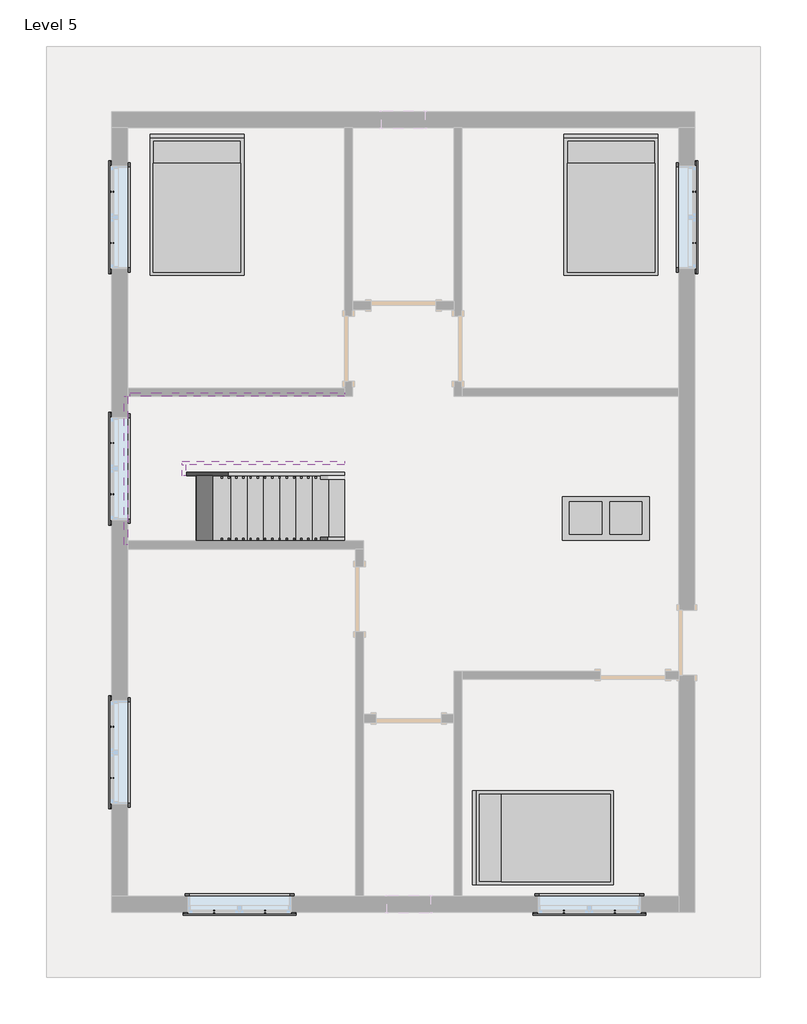
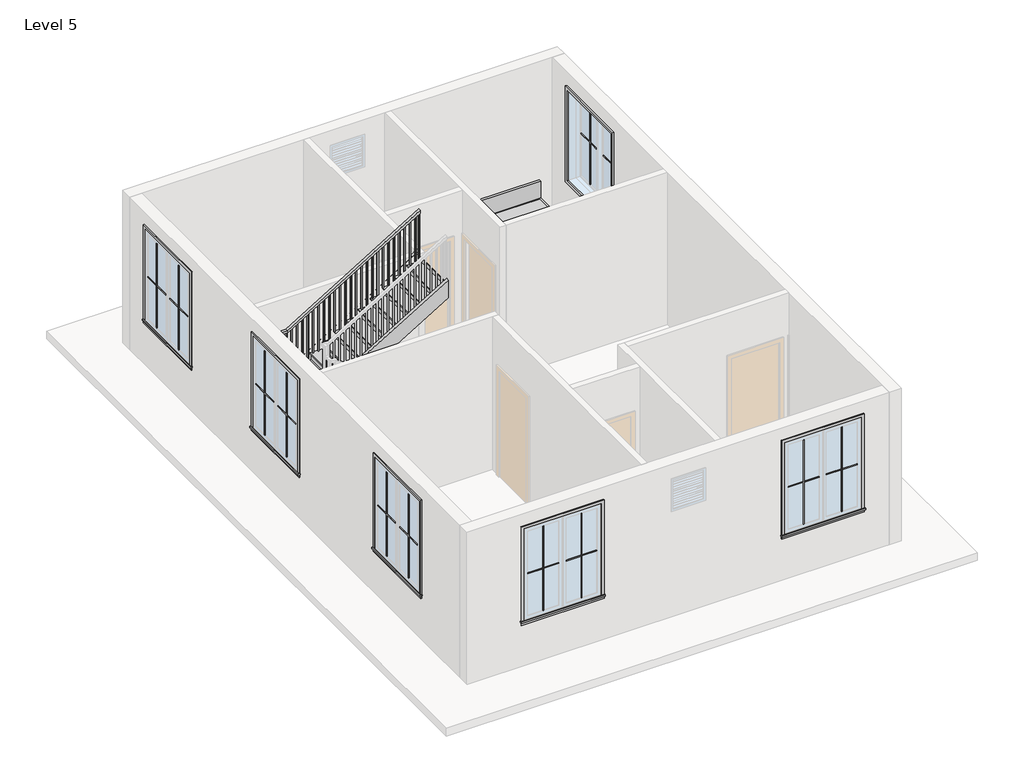
# One storey, part 2 of 2: 25 proxies, 6 members, 3 furniture elements, 1 railing, 1 stair flight.
"""IFC4 building model written with IfcOpenShell, lengths in millimetres."""

from ifc_helpers import new_model, si_unit, frame, origin, place, context, project, spatial, polyline, outline, extrude, faceted_brep, transform, mapped, element, save
from components import muntin_pattern_2x2_muntin_pattern_2x2_bff912c5, muntin_pattern_2x2_muntin_pattern_2x2_c2194282, trim_window_exterior_flat_with_sill_e04b3088, trim_window_interior_flat_picture_frame_2a7685fe, coffee_table_with_brass_mullions_11320_coffee_table_with_5962bef7, bed_17739_bed_17739_15c61121, stair_flight_f9c943de

model = new_model("IFC4")

# Units and contexts
model_context = context("Model", 3, world=origin())
ifc_project = project(units=[si_unit("LENGTHUNIT", "METRE", prefix="MILLI")], contexts=[model_context])

# Site, building, storey
site = spatial("IfcSite", under=ifc_project)
building = spatial("IfcBuilding", under=site)
storey = spatial("IfcBuildingStorey", under=building, Name="Level 5", Elevation=9601.2)

# Proxies
placement = place(None, origin())
muntin_pattern_2x2_muntin_pattern_2x2_shape = muntin_pattern_2x2_muntin_pattern_2x2_bff912c5(model_context)
element("IfcBuildingElementProxy", 1, Name="Muntin Pattern_2x2 : Muntin Pattern_2x2", ObjectType="Muntin Pattern_2x2 : Muntin Pattern_2x2", at=placement, inside=storey, context=model_context, shape_type="MappedRepresentation", body=[
    mapped(muntin_pattern_2x2_muntin_pattern_2x2_shape, transform((-3196.8535855, -5792.3946383, 10585.45), x_axis=(-1.0, 0.0, 0.0), y_axis=(0.0, -1.0, 0.0), z_axis=(0.0, 0.0, 1.0))),
])
element("IfcBuildingElementProxy", 2, Name="Muntin Pattern_2x2 : Muntin Pattern_2x2", ObjectType="Muntin Pattern_2x2 : Muntin Pattern_2x2", at=placement, inside=storey, context=model_context, shape_type="MappedRepresentation", body=[
    mapped(muntin_pattern_2x2_muntin_pattern_2x2_shape, transform((-5347.9160855, -3914.3821383, 10585.45), x_axis=(0.0, 1.0, 0.0), y_axis=(-1.0, 0.0, 0.0), z_axis=(0.0, 0.0, 1.0))),
])
element("IfcBuildingElementProxy", 3, Name="Muntin Pattern_2x2 : Muntin Pattern_2x2", ObjectType="Muntin Pattern_2x2 : Muntin Pattern_2x2", at=placement, inside=storey, context=model_context, shape_type="MappedRepresentation", body=[
    mapped(muntin_pattern_2x2_muntin_pattern_2x2_shape, transform((1721.2214145, -5792.3946383, 10585.45), x_axis=(-1.0, 0.0, 0.0), y_axis=(0.0, -1.0, 0.0), z_axis=(0.0, 0.0, 1.0))),
])
element("IfcBuildingElementProxy", 4, Name="Muntin Pattern_2x2 : Muntin Pattern_2x2", ObjectType="Muntin Pattern_2x2 : Muntin Pattern_2x2", at=placement, inside=storey, context=model_context, shape_type="MappedRepresentation", body=[
    mapped(muntin_pattern_2x2_muntin_pattern_2x2_shape, transform((2837.2339145, 4324.7428617, 10585.45), x_axis=(0.0, -1.0, 0.0), y_axis=(1.0, 0.0, 0.0), z_axis=(0.0, 0.0, 1.0))),
])
element("IfcBuildingElementProxy", 5, Name="Muntin Pattern_2x2 : Muntin Pattern_2x2", ObjectType="Muntin Pattern_2x2 : Muntin Pattern_2x2", at=placement, inside=storey, context=model_context, shape_type="MappedRepresentation", body=[
    mapped(muntin_pattern_2x2_muntin_pattern_2x2_shape, transform((-5347.9160855, 3604.0178617, 10585.45), x_axis=(0.0, 1.0, 0.0), y_axis=(-1.0, 0.0, 0.0), z_axis=(0.0, 0.0, 1.0))),
])
element("IfcBuildingElementProxy", 6, Name="Muntin Pattern_2x2 : Muntin Pattern_2x2", ObjectType="Muntin Pattern_2x2 : Muntin Pattern_2x2", at=placement, inside=storey, context=model_context, shape_type="MappedRepresentation", body=[
    mapped(muntin_pattern_2x2_muntin_pattern_2x2_shape, transform((-5347.9160855, 73.4178617, 10585.45), x_axis=(0.0, 1.0, 0.0), y_axis=(-1.0, 0.0, 0.0), z_axis=(0.0, 0.0, 1.0))),
])
muntin_pattern_2x2_muntin_pattern_2x2_2_shape = muntin_pattern_2x2_muntin_pattern_2x2_c2194282(model_context)
element("IfcBuildingElementProxy", 7, Name="Muntin Pattern_2x2 : Muntin Pattern_2x2", ObjectType="Muntin Pattern_2x2 : Muntin Pattern_2x2", at=placement, inside=storey, context=model_context, shape_type="MappedRepresentation", body=[
    mapped(muntin_pattern_2x2_muntin_pattern_2x2_2_shape, transform((-3917.5785855, -5792.3946383, 10585.45), x_axis=(1.0, 0.0, 0.0), y_axis=(0.0, 1.0, 0.0), z_axis=(0.0, 0.0, 1.0))),
])
element("IfcBuildingElementProxy", 8, Name="Muntin Pattern_2x2 : Muntin Pattern_2x2", ObjectType="Muntin Pattern_2x2 : Muntin Pattern_2x2", at=placement, inside=storey, context=model_context, shape_type="MappedRepresentation", body=[
    mapped(muntin_pattern_2x2_muntin_pattern_2x2_2_shape, transform((-5347.9160855, -3193.6571383, 10585.45), x_axis=(0.0, -1.0, 0.0), y_axis=(1.0, 0.0, 0.0), z_axis=(0.0, 0.0, 1.0))),
])
element("IfcBuildingElementProxy", 9, Name="Muntin Pattern_2x2 : Muntin Pattern_2x2", ObjectType="Muntin Pattern_2x2 : Muntin Pattern_2x2", at=placement, inside=storey, context=model_context, shape_type="MappedRepresentation", body=[
    mapped(muntin_pattern_2x2_muntin_pattern_2x2_2_shape, transform((1000.4964145, -5792.3946383, 10585.45), x_axis=(1.0, 0.0, 0.0), y_axis=(0.0, 1.0, 0.0), z_axis=(0.0, 0.0, 1.0))),
])
element("IfcBuildingElementProxy", 10, Name="Muntin Pattern_2x2 : Muntin Pattern_2x2", ObjectType="Muntin Pattern_2x2 : Muntin Pattern_2x2", at=placement, inside=storey, context=model_context, shape_type="MappedRepresentation", body=[
    mapped(muntin_pattern_2x2_muntin_pattern_2x2_2_shape, transform((2837.2339145, 3604.0178617, 10585.45), x_axis=(0.0, 1.0, 0.0), y_axis=(-1.0, 0.0, 0.0), z_axis=(0.0, 0.0, 1.0))),
])
element("IfcBuildingElementProxy", 11, Name="Muntin Pattern_2x2 : Muntin Pattern_2x2", ObjectType="Muntin Pattern_2x2 : Muntin Pattern_2x2", at=placement, inside=storey, context=model_context, shape_type="MappedRepresentation", body=[
    mapped(muntin_pattern_2x2_muntin_pattern_2x2_2_shape, transform((-5347.9160855, 4324.7428617, 10585.45), x_axis=(0.0, -1.0, 0.0), y_axis=(1.0, 0.0, 0.0), z_axis=(0.0, 0.0, 1.0))),
])
element("IfcBuildingElementProxy", 12, Name="Muntin Pattern_2x2 : Muntin Pattern_2x2", ObjectType="Muntin Pattern_2x2 : Muntin Pattern_2x2", at=placement, inside=storey, context=model_context, shape_type="MappedRepresentation", body=[
    mapped(muntin_pattern_2x2_muntin_pattern_2x2_2_shape, transform((-5347.9160855, 794.1428617, 10585.45), x_axis=(0.0, -1.0, 0.0), y_axis=(1.0, 0.0, 0.0), z_axis=(0.0, 0.0, 1.0))),
])
trim_window_exterior_flat_with_sill_shape = trim_window_exterior_flat_with_sill_e04b3088(model_context)
element("IfcBuildingElementProxy", 13, Name="Trim-Window-Exterior-Flat : with Sill", ObjectType="Trim-Window-Exterior-Flat : with Sill", at=placement, inside=storey, context=model_context, shape_type="MappedRepresentation", body=[
    mapped(trim_window_exterior_flat_with_sill_shape, transform((-3557.2160855, -5801.9196383, 12344.4), x_axis=(1.0, 0.0, 0.0), y_axis=(0.0, 0.0, 1.0), z_axis=(0.0, -1.0, 0.0))),
])
element("IfcBuildingElementProxy", 14, Name="Trim-Window-Exterior-Flat : with Sill", ObjectType="Trim-Window-Exterior-Flat : with Sill", at=placement, inside=storey, context=model_context, shape_type="MappedRepresentation", body=[
    mapped(trim_window_exterior_flat_with_sill_shape, transform((-5357.4410855, -3554.0196383, 12344.4), x_axis=(0.0, -1.0, 0.0), y_axis=(0.0, 0.0, 1.0), z_axis=(-1.0, 0.0, 0.0))),
])
element("IfcBuildingElementProxy", 15, Name="Trim-Window-Exterior-Flat : with Sill", ObjectType="Trim-Window-Exterior-Flat : with Sill", at=placement, inside=storey, context=model_context, shape_type="MappedRepresentation", body=[
    mapped(trim_window_exterior_flat_with_sill_shape, transform((1360.8589145, -5801.9196383, 12344.4), x_axis=(1.0, 0.0, 0.0), y_axis=(0.0, 0.0, 1.0), z_axis=(0.0, -1.0, 0.0))),
])
element("IfcBuildingElementProxy", 16, Name="Trim-Window-Exterior-Flat : with Sill", ObjectType="Trim-Window-Exterior-Flat : with Sill", at=placement, inside=storey, context=model_context, shape_type="MappedRepresentation", body=[
    mapped(trim_window_exterior_flat_with_sill_shape, transform((2846.7589145, 3964.3803617, 12344.4), x_axis=(0.0, 1.0, 0.0), y_axis=(0.0, 0.0, 1.0), z_axis=(1.0, 0.0, 0.0))),
])
element("IfcBuildingElementProxy", 17, Name="Trim-Window-Exterior-Flat : with Sill", ObjectType="Trim-Window-Exterior-Flat : with Sill", at=placement, inside=storey, context=model_context, shape_type="MappedRepresentation", body=[
    mapped(trim_window_exterior_flat_with_sill_shape, transform((-5357.4410855, 3964.3803617, 12344.4), x_axis=(0.0, -1.0, 0.0), y_axis=(0.0, 0.0, 1.0), z_axis=(-1.0, 0.0, 0.0))),
])
element("IfcBuildingElementProxy", 18, Name="Trim-Window-Exterior-Flat : with Sill", ObjectType="Trim-Window-Exterior-Flat : with Sill", at=placement, inside=storey, context=model_context, shape_type="MappedRepresentation", body=[
    mapped(trim_window_exterior_flat_with_sill_shape, transform((-5357.4410855, 433.7803617, 12344.4), x_axis=(0.0, -1.0, 0.0), y_axis=(0.0, 0.0, 1.0), z_axis=(-1.0, 0.0, 0.0))),
])
trim_window_interior_flat_picture_frame_shape = trim_window_interior_flat_picture_frame_2a7685fe(model_context)
element("IfcBuildingElementProxy", 19, Name="Trim-Window-Interior-Flat : Picture Frame", ObjectType="Trim-Window-Interior-Flat : Picture Frame", at=placement, inside=storey, context=model_context, shape_type="MappedRepresentation", body=[
    mapped(trim_window_interior_flat_picture_frame_shape, transform((-3557.2160855, -5573.3196383, 12344.4), x_axis=(-1.0, 0.0, 0.0), y_axis=(0.0, 0.0, 1.0), z_axis=(0.0, 1.0, 0.0))),
])
element("IfcBuildingElementProxy", 20, Name="Trim-Window-Interior-Flat : Picture Frame", ObjectType="Trim-Window-Interior-Flat : Picture Frame", at=placement, inside=storey, context=model_context, shape_type="MappedRepresentation", body=[
    mapped(trim_window_interior_flat_picture_frame_shape, transform((-5128.8410855, -3554.0196383, 12344.4), x_axis=(0.0, 1.0, 0.0), y_axis=(0.0, 0.0, 1.0), z_axis=(1.0, 0.0, 0.0))),
])
element("IfcBuildingElementProxy", 21, Name="Trim-Window-Interior-Flat : Picture Frame", ObjectType="Trim-Window-Interior-Flat : Picture Frame", at=placement, inside=storey, context=model_context, shape_type="MappedRepresentation", body=[
    mapped(trim_window_interior_flat_picture_frame_shape, transform((1360.8589145, -5573.3196383, 12344.4), x_axis=(-1.0, 0.0, 0.0), y_axis=(0.0, 0.0, 1.0), z_axis=(0.0, 1.0, 0.0))),
])
element("IfcBuildingElementProxy", 22, Name="Trim-Window-Interior-Flat : Picture Frame", ObjectType="Trim-Window-Interior-Flat : Picture Frame", at=placement, inside=storey, context=model_context, shape_type="MappedRepresentation", body=[
    mapped(trim_window_interior_flat_picture_frame_shape, transform((2618.1589145, 3964.3803617, 12344.4), x_axis=(0.0, -1.0, 0.0), y_axis=(0.0, 0.0, 1.0), z_axis=(-1.0, 0.0, 0.0))),
])
element("IfcBuildingElementProxy", 23, Name="Trim-Window-Interior-Flat : Picture Frame", ObjectType="Trim-Window-Interior-Flat : Picture Frame", at=placement, inside=storey, context=model_context, shape_type="MappedRepresentation", body=[
    mapped(trim_window_interior_flat_picture_frame_shape, transform((-5128.8410855, 3964.3803617, 12344.4), x_axis=(0.0, 1.0, 0.0), y_axis=(0.0, 0.0, 1.0), z_axis=(1.0, 0.0, 0.0))),
])
element("IfcBuildingElementProxy", 24, Name="Trim-Window-Interior-Flat : Picture Frame", ObjectType="Trim-Window-Interior-Flat : Picture Frame", at=placement, inside=storey, context=model_context, shape_type="MappedRepresentation", body=[
    mapped(trim_window_interior_flat_picture_frame_shape, transform((-5128.8410855, 433.7803617, 12344.4), x_axis=(0.0, 1.0, 0.0), y_axis=(0.0, 0.0, 1.0), z_axis=(1.0, 0.0, 0.0))),
])
coffee_table_with_brass_mullions_11320_coffee_table_with_shape = coffee_table_with_brass_mullions_11320_coffee_table_with_5962bef7(model_context)
element("IfcBuildingElementProxy", 25, Name="coffee_table_with_brass_mullions_11320 : coffee_table_with_brass_mullions_11320", ObjectType="coffee_table_with_brass_mullions_11320 : coffee_table_with_brass_mullions_11320", at=placement, inside=storey, context=model_context, shape_type="MappedRepresentation", body=[
    mapped(coffee_table_with_brass_mullions_11320_coffee_table_with_shape, transform((2229.2258874, -696.5196383, 9601.2), x_axis=(1.0, 0.0, 0.0), y_axis=(0.0, 1.0, 0.0), z_axis=(0.0, 0.0, 1.0))),
])

# Furniture
bed_17739_bed_17739_shape = bed_17739_bed_17739_15c61121(model_context)
element("IfcFurniture", 26, ObjectType="Bed_17739 : Bed_17739", at=placement, inside=storey, context=model_context, shape_type="MappedRepresentation", body=[
    mapped(bed_17739_bed_17739_shape, transform((1665.6589145, 4116.7803617, 9601.2), x_axis=(1.0, 0.0, 0.0), y_axis=(0.0, 1.0, 0.0), z_axis=(0.0, 0.0, 1.0))),
])
element("IfcFurniture", 27, ObjectType="Bed_17739 : Bed_17739", at=placement, inside=storey, context=model_context, shape_type="MappedRepresentation", body=[
    mapped(bed_17739_bed_17739_shape, transform((-4157.2910855, 4116.7803617, 9601.2), x_axis=(1.0, 0.0, 0.0), y_axis=(0.0, 1.0, 0.0), z_axis=(0.0, 0.0, 1.0))),
])
element("IfcFurniture", 28, ObjectType="Bed_17739 : Bed_17739", at=placement, inside=storey, context=model_context, shape_type="MappedRepresentation", body=[
    mapped(bed_17739_bed_17739_shape, transform((732.2089145, -4754.5725945, 9601.2), x_axis=(0.0, 1.0, 0.0), y_axis=(-1.0, 0.0, 0.0), z_axis=(0.0, 0.0, 1.0))),
])

# Members
element("IfcMember", 29, ObjectType="Stringer - 2\" Width", at=placement, inside=storey, context=model_context, shape_type="SweptSolid", body=[
    extrude(outline(polyline([(9601.2, -2080.8410855), (9813.314512, -2080.8410855), (11201.4, -4371.1821407), (11201.4, -4959.2565972), (9601.2, -2318.9265972), (9601.2, -2080.8410855)])), frame((0.0, -633.0196383, 0.0), z_axis=(0.0, 1.0, 0.0), x_axis=(0.0, 0.0, 1.0)), (0.0, 0.0, 1.0), 50.8),
])
element("IfcMember", 30, ObjectType="Stringer - 2\" Width", at=placement, inside=storey, context=model_context, shape_type="SweptSolid", body=[
    extrude(outline(polyline([(-5128.8410855, -633.0196383), (-5179.6410855, -633.0196383), (-5179.6410855, 1449.7803617), (-5128.8410855, 1449.7803617), (-5128.8410855, -633.0196383)])), frame((0.0, 0.0, 10896.6), z_axis=(0.0, 0.0, 1.0), x_axis=(1.0, 0.0, 0.0)), (0.0, 0.0, 1.0), 304.8),
])
element("IfcMember", 31, ObjectType="Stringer - 2\" Width", at=placement, inside=storey, context=model_context, shape_type="SweptSolid", body=[
    extrude(outline(polyline([(10896.6, -4505.9455737), (12366.3602959, -2080.8410855), (12722.7690574, -2080.8410855), (10896.6, -5094.0200302), (10896.6, -4505.9455737)])), frame((0.0, 1449.7803617, 0.0), z_axis=(0.0, 1.0, 0.0), x_axis=(0.0, 0.0, 1.0)), (0.0, 0.0, 1.0), 50.8),
])
element("IfcMember", 32, ObjectType="Stringer - 2\" Width", at=placement, inside=storey, context=model_context, shape_type="SweptSolid", body=[
    extrude(outline(polyline([(9601.2, -2080.8410855), (9813.314512, -2080.8410855), (11167.9811786, -4316.0410855), (10811.5724171, -4316.0410855), (9601.2, -2318.9265972), (9601.2, -2080.8410855)])), frame((0.0, 332.1803617, 0.0), z_axis=(0.0, 1.0, 0.0), x_axis=(0.0, 0.0, 1.0)), (0.0, 0.0, 1.0), 50.8),
])
element("IfcMember", 33, ObjectType="Stringer - 2\" Width", at=placement, inside=storey, context=model_context, shape_type="SweptSolid", body=[
    extrude(outline(polyline([(-4316.0410855, 332.1803617), (-4366.8410855, 332.1803617), (-4366.8410855, 484.5803617), (-4316.0410855, 484.5803617), (-4316.0410855, 332.1803617)])), frame((0.0, 0.0, 10896.6), z_axis=(0.0, 0.0, 1.0), x_axis=(1.0, 0.0, 0.0)), (0.0, 0.0, 1.0), 304.8),
])
element("IfcMember", 34, ObjectType="Stringer - 2\" Width", at=placement, inside=storey, context=model_context, shape_type="SweptSolid", body=[
    extrude(outline(polyline([(11337.314512, -4366.8410855), (10980.9057504, -4366.8410855), (12366.3602959, -2080.8410855), (12722.7690574, -2080.8410855), (11337.314512, -4366.8410855)])), frame((0.0, 484.5803617, 0.0), z_axis=(0.0, 1.0, 0.0), x_axis=(0.0, 0.0, 1.0)), (0.0, 0.0, 1.0), 50.8),
])

# Railing
element("IfcRailing", 35, ObjectType="Handrail - Rectangular", at=placement, inside=storey, context=model_context, shape_type="SolidModel", body=[
    faceted_brep([(-2080.8410855, -582.2196383, 10654.1454545), (-2080.8410855, -582.2196383, 10594.7439943), (-2080.8410855, -531.4196383, 10594.7439943), (-2080.8410855, -531.4196383, 10654.1454545), (-4366.8410855, -582.2196383, 12039.6), (-4381.0334949, -582.2196383, 11988.8), (-4381.0334949, -531.4196383, 11988.8), (-4366.8410855, -531.4196383, 12039.6), (-5128.8410855, -582.2196383, 12039.6), (-5128.8410855, -582.2196383, 11988.8), (-5078.0410855, -531.4196383, 11988.8), (-5078.0410855, -531.4196383, 12039.6), (-5128.8410855, 1449.7803617, 12039.6), (-5128.8410855, 1449.7803617, 11988.8), (-5078.0410855, 1398.9803617, 11988.8), (-5078.0410855, 1398.9803617, 12039.6), (-4595.4410855, 1449.7803617, 12039.6), (-4581.2486761, 1449.7803617, 11988.8), (-4581.2486761, 1398.9803617, 11988.8), (-4595.4410855, 1398.9803617, 12039.6), (-2080.8410855, 1449.7803617, 13563.6), (-2080.8410855, 1398.9803617, 13563.6), (-2080.8410855, 1398.9803617, 13504.1985397), (-2080.8410855, 1449.7803617, 13504.1985397)], [[[0, 1, 2, 3]], [[1, 0, 4, 5]], [[2, 1, 5, 6]], [[3, 2, 6, 7]], [[0, 3, 7, 4]], [[5, 4, 8, 9]], [[6, 5, 9, 10]], [[7, 6, 10, 11]], [[4, 7, 11, 8]], [[9, 8, 12, 13]], [[10, 9, 13, 14]], [[11, 10, 14, 15]], [[8, 11, 15, 12]], [[13, 12, 16, 17]], [[14, 13, 17, 18]], [[15, 14, 18, 19]], [[12, 15, 19, 16]], [[20, 21, 22, 23]], [[17, 16, 20, 23]], [[18, 17, 23, 22]], [[19, 18, 22, 21]], [[16, 19, 21, 20]]]),
    extrude(outline(polyline([(13452.2439943, -2166.5660855), (12510.6545455, -2166.5660855), (12510.6545455, -2147.5160855), (13463.7894488, -2147.5160855), (13452.2439943, -2166.5660855)])), frame((0.0, 1414.8553617, 0.0), z_axis=(0.0, 1.0, 0.0), x_axis=(0.0, 0.0, 1.0)), (0.0, 0.0, 1.0), 19.05),
    extrude(outline(polyline([(13390.6682367, -2268.1660855), (12510.6545455, -2268.1660855), (12510.6545455, -2249.1160855), (13402.2136913, -2249.1160855), (13390.6682367, -2268.1660855)])), frame((0.0, 1414.8553617, 0.0), z_axis=(0.0, 1.0, 0.0), x_axis=(0.0, 0.0, 1.0)), (0.0, 0.0, 1.0), 19.05),
    extrude(outline(polyline([(13329.0924791, -2369.7660855), (12372.1090909, -2369.7660855), (12372.1090909, -2350.7160855), (13340.6379337, -2350.7160855), (13329.0924791, -2369.7660855)])), frame((0.0, 1414.8553617, 0.0), z_axis=(0.0, 1.0, 0.0), x_axis=(0.0, 0.0, 1.0)), (0.0, 0.0, 1.0), 19.05),
    extrude(outline(polyline([(13267.5167216, -2471.3660855), (12372.1090909, -2471.3660855), (12372.1090909, -2452.3160855), (13279.0621761, -2452.3160855), (13267.5167216, -2471.3660855)])), frame((0.0, 1414.8553617, 0.0), z_axis=(0.0, 1.0, 0.0), x_axis=(0.0, 0.0, 1.0)), (0.0, 0.0, 1.0), 19.05),
    extrude(outline(polyline([(13205.940964, -2572.9660855), (12233.5636364, -2572.9660855), (12233.5636364, -2553.9160855), (13217.4864185, -2553.9160855), (13205.940964, -2572.9660855)])), frame((0.0, 1414.8553617, 0.0), z_axis=(0.0, 1.0, 0.0), x_axis=(0.0, 0.0, 1.0)), (0.0, 0.0, 1.0), 19.05),
    extrude(outline(polyline([(13144.3652064, -2674.5660855), (12233.5636364, -2674.5660855), (12233.5636364, -2655.5160855), (13155.910661, -2655.5160855), (13144.3652064, -2674.5660855)])), frame((0.0, 1414.8553617, 0.0), z_axis=(0.0, 1.0, 0.0), x_axis=(0.0, 0.0, 1.0)), (0.0, 0.0, 1.0), 19.05),
    extrude(outline(polyline([(13082.7894488, -2776.1660855), (12233.5636364, -2776.1660855), (12233.5636364, -2757.1160855), (13094.3349034, -2757.1160855), (13082.7894488, -2776.1660855)])), frame((0.0, 1414.8553617, 0.0), z_axis=(0.0, 1.0, 0.0), x_axis=(0.0, 0.0, 1.0)), (0.0, 0.0, 1.0), 19.05),
    extrude(outline(polyline([(13021.2136913, -2877.7660855), (12095.0181818, -2877.7660855), (12095.0181818, -2858.7160855), (13032.7591458, -2858.7160855), (13021.2136913, -2877.7660855)])), frame((0.0, 1414.8553617, 0.0), z_axis=(0.0, 1.0, 0.0), x_axis=(0.0, 0.0, 1.0)), (0.0, 0.0, 1.0), 19.05),
    extrude(outline(polyline([(12959.6379337, -2979.3660855), (12095.0181818, -2979.3660855), (12095.0181818, -2960.3160855), (12971.1833882, -2960.3160855), (12959.6379337, -2979.3660855)])), frame((0.0, 1414.8553617, 0.0), z_axis=(0.0, 1.0, 0.0), x_axis=(0.0, 0.0, 1.0)), (0.0, 0.0, 1.0), 19.05),
    extrude(outline(polyline([(12898.0621761, -3080.9660855), (11956.4727273, -3080.9660855), (11956.4727273, -3061.9160855), (12909.6076307, -3061.9160855), (12898.0621761, -3080.9660855)])), frame((0.0, 1414.8553617, 0.0), z_axis=(0.0, 1.0, 0.0), x_axis=(0.0, 0.0, 1.0)), (0.0, 0.0, 1.0), 19.05),
    extrude(outline(polyline([(12836.4864185, -3182.5660855), (11956.4727273, -3182.5660855), (11956.4727273, -3163.5160855), (12848.0318731, -3163.5160855), (12836.4864185, -3182.5660855)])), frame((0.0, 1414.8553617, 0.0), z_axis=(0.0, 1.0, 0.0), x_axis=(0.0, 0.0, 1.0)), (0.0, 0.0, 1.0), 19.05),
    extrude(outline(polyline([(12774.910661, -3284.1660855), (11817.9272727, -3284.1660855), (11817.9272727, -3265.1160855), (12786.4561155, -3265.1160855), (12774.910661, -3284.1660855)])), frame((0.0, 1414.8553617, 0.0), z_axis=(0.0, 1.0, 0.0), x_axis=(0.0, 0.0, 1.0)), (0.0, 0.0, 1.0), 19.05),
    extrude(outline(polyline([(12713.3349034, -3385.7660855), (11817.9272727, -3385.7660855), (11817.9272727, -3366.7160855), (12724.8803579, -3366.7160855), (12713.3349034, -3385.7660855)])), frame((0.0, 1414.8553617, 0.0), z_axis=(0.0, 1.0, 0.0), x_axis=(0.0, 0.0, 1.0)), (0.0, 0.0, 1.0), 19.05),
    extrude(outline(polyline([(12651.7591458, -3487.3660855), (11679.3818182, -3487.3660855), (11679.3818182, -3468.3160855), (12663.3046004, -3468.3160855), (12651.7591458, -3487.3660855)])), frame((0.0, 1414.8553617, 0.0), z_axis=(0.0, 1.0, 0.0), x_axis=(0.0, 0.0, 1.0)), (0.0, 0.0, 1.0), 19.05),
    extrude(outline(polyline([(12590.1833882, -3588.9660855), (11679.3818182, -3588.9660855), (11679.3818182, -3569.9160855), (12601.7288428, -3569.9160855), (12590.1833882, -3588.9660855)])), frame((0.0, 1414.8553617, 0.0), z_axis=(0.0, 1.0, 0.0), x_axis=(0.0, 0.0, 1.0)), (0.0, 0.0, 1.0), 19.05),
    extrude(outline(polyline([(12528.6076307, -3690.5660855), (11679.3818182, -3690.5660855), (11679.3818182, -3671.5160855), (12540.1530852, -3671.5160855), (12528.6076307, -3690.5660855)])), frame((0.0, 1414.8553617, 0.0), z_axis=(0.0, 1.0, 0.0), x_axis=(0.0, 0.0, 1.0)), (0.0, 0.0, 1.0), 19.05),
    extrude(outline(polyline([(12467.0318731, -3792.1660855), (11540.8363636, -3792.1660855), (11540.8363636, -3773.1160855), (12478.5773276, -3773.1160855), (12467.0318731, -3792.1660855)])), frame((0.0, 1414.8553617, 0.0), z_axis=(0.0, 1.0, 0.0), x_axis=(0.0, 0.0, 1.0)), (0.0, 0.0, 1.0), 19.05),
    extrude(outline(polyline([(12405.4561155, -3893.7660855), (11540.8363636, -3893.7660855), (11540.8363636, -3874.7160855), (12417.00157, -3874.7160855), (12405.4561155, -3893.7660855)])), frame((0.0, 1414.8553617, 0.0), z_axis=(0.0, 1.0, 0.0), x_axis=(0.0, 0.0, 1.0)), (0.0, 0.0, 1.0), 19.05),
    extrude(outline(polyline([(12343.8803579, -3995.3660855), (11402.2909091, -3995.3660855), (11402.2909091, -3976.3160855), (12355.4258125, -3976.3160855), (12343.8803579, -3995.3660855)])), frame((0.0, 1414.8553617, 0.0), z_axis=(0.0, 1.0, 0.0), x_axis=(0.0, 0.0, 1.0)), (0.0, 0.0, 1.0), 19.05),
    extrude(outline(polyline([(12282.3046004, -4096.9660855), (11402.2909091, -4096.9660855), (11402.2909091, -4077.9160855), (12293.8500549, -4077.9160855), (12282.3046004, -4096.9660855)])), frame((0.0, 1414.8553617, 0.0), z_axis=(0.0, 1.0, 0.0), x_axis=(0.0, 0.0, 1.0)), (0.0, 0.0, 1.0), 19.05),
    extrude(outline(polyline([(12220.7288428, -4198.5660855), (11263.7454545, -4198.5660855), (11263.7454545, -4179.5160855), (12232.2742973, -4179.5160855), (12220.7288428, -4198.5660855)])), frame((0.0, 1414.8553617, 0.0), z_axis=(0.0, 1.0, 0.0), x_axis=(0.0, 0.0, 1.0)), (0.0, 0.0, 1.0), 19.05),
    extrude(outline(polyline([(12159.1530852, -4300.1660855), (11263.7454545, -4300.1660855), (11263.7454545, -4281.1160855), (12170.6985397, -4281.1160855), (12159.1530852, -4300.1660855)])), frame((0.0, 1414.8553617, 0.0), z_axis=(0.0, 1.0, 0.0), x_axis=(0.0, 0.0, 1.0)), (0.0, 0.0, 1.0), 19.05),
    extrude(outline(polyline([(12097.5773276, -4401.7660855), (11125.2, -4401.7660855), (11125.2, -4382.7160855), (12109.1227822, -4382.7160855), (12097.5773276, -4401.7660855)])), frame((0.0, 1414.8553617, 0.0), z_axis=(0.0, 1.0, 0.0), x_axis=(0.0, 0.0, 1.0)), (0.0, 0.0, 1.0), 19.05),
    extrude(outline(polyline([(12036.00157, -4503.3660855), (11125.2, -4503.3660855), (11125.2, -4484.3160855), (12047.5470246, -4484.3160855), (12036.00157, -4503.3660855)])), frame((0.0, 1414.8553617, 0.0), z_axis=(0.0, 1.0, 0.0), x_axis=(0.0, 0.0, 1.0)), (0.0, 0.0, 1.0), 19.05),
    extrude(outline(polyline([(-4604.9660855, 1433.9053617), (-4585.9160855, 1433.9053617), (-4585.9160855, 1414.8553617), (-4604.9660855, 1414.8553617), (-4604.9660855, 1433.9053617)])), frame((0.0, 0.0, 11125.2), z_axis=(0.0, 0.0, 1.0), x_axis=(1.0, 0.0, 0.0)), (0.0, 0.0, 1.0), 863.6),
    extrude(outline(polyline([(-4706.5660855, 1433.9053617), (-4687.5160855, 1433.9053617), (-4687.5160855, 1414.8553617), (-4706.5660855, 1414.8553617), (-4706.5660855, 1433.9053617)])), frame((0.0, 0.0, 11125.2), z_axis=(0.0, 0.0, 1.0), x_axis=(1.0, 0.0, 0.0)), (0.0, 0.0, 1.0), 863.6),
    extrude(outline(polyline([(-4808.1660855, 1433.9053617), (-4789.1160855, 1433.9053617), (-4789.1160855, 1414.8553617), (-4808.1660855, 1414.8553617), (-4808.1660855, 1433.9053617)])), frame((0.0, 0.0, 11125.2), z_axis=(0.0, 0.0, 1.0), x_axis=(1.0, 0.0, 0.0)), (0.0, 0.0, 1.0), 863.6),
    extrude(outline(polyline([(-4909.7660855, 1433.9053617), (-4890.7160855, 1433.9053617), (-4890.7160855, 1414.8553617), (-4909.7660855, 1414.8553617), (-4909.7660855, 1433.9053617)])), frame((0.0, 0.0, 11125.2), z_axis=(0.0, 0.0, 1.0), x_axis=(1.0, 0.0, 0.0)), (0.0, 0.0, 1.0), 863.6),
    extrude(outline(polyline([(-5011.3660855, 1433.9053617), (-4992.3160855, 1433.9053617), (-4992.3160855, 1414.8553617), (-5011.3660855, 1414.8553617), (-5011.3660855, 1433.9053617)])), frame((0.0, 0.0, 11125.2), z_axis=(0.0, 0.0, 1.0), x_axis=(1.0, 0.0, 0.0)), (0.0, 0.0, 1.0), 863.6),
    extrude(outline(polyline([(-5112.9660855, 1364.0553617), (-5112.9660855, 1383.1053617), (-5093.9160855, 1383.1053617), (-5093.9160855, 1364.0553617), (-5112.9660855, 1364.0553617)])), frame((0.0, 0.0, 11125.2), z_axis=(0.0, 0.0, 1.0), x_axis=(1.0, 0.0, 0.0)), (0.0, 0.0, 1.0), 863.6),
    extrude(outline(polyline([(-5112.9660855, 1262.4553617), (-5112.9660855, 1281.5053617), (-5093.9160855, 1281.5053617), (-5093.9160855, 1262.4553617), (-5112.9660855, 1262.4553617)])), frame((0.0, 0.0, 11125.2), z_axis=(0.0, 0.0, 1.0), x_axis=(1.0, 0.0, 0.0)), (0.0, 0.0, 1.0), 863.6),
    extrude(outline(polyline([(-5112.9660855, 1160.8553617), (-5112.9660855, 1179.9053617), (-5093.9160855, 1179.9053617), (-5093.9160855, 1160.8553617), (-5112.9660855, 1160.8553617)])), frame((0.0, 0.0, 11125.2), z_axis=(0.0, 0.0, 1.0), x_axis=(1.0, 0.0, 0.0)), (0.0, 0.0, 1.0), 863.6),
    extrude(outline(polyline([(-5112.9660855, 1059.2553617), (-5112.9660855, 1078.3053617), (-5093.9160855, 1078.3053617), (-5093.9160855, 1059.2553617), (-5112.9660855, 1059.2553617)])), frame((0.0, 0.0, 11125.2), z_axis=(0.0, 0.0, 1.0), x_axis=(1.0, 0.0, 0.0)), (0.0, 0.0, 1.0), 863.6),
    extrude(outline(polyline([(-5112.9660855, 957.6553617), (-5112.9660855, 976.7053617), (-5093.9160855, 976.7053617), (-5093.9160855, 957.6553617), (-5112.9660855, 957.6553617)])), frame((0.0, 0.0, 11125.2), z_axis=(0.0, 0.0, 1.0), x_axis=(1.0, 0.0, 0.0)), (0.0, 0.0, 1.0), 863.6),
    extrude(outline(polyline([(-5112.9660855, 856.0553617), (-5112.9660855, 875.1053617), (-5093.9160855, 875.1053617), (-5093.9160855, 856.0553617), (-5112.9660855, 856.0553617)])), frame((0.0, 0.0, 11125.2), z_axis=(0.0, 0.0, 1.0), x_axis=(1.0, 0.0, 0.0)), (0.0, 0.0, 1.0), 863.6),
    extrude(outline(polyline([(-5112.9660855, 754.4553617), (-5112.9660855, 773.5053617), (-5093.9160855, 773.5053617), (-5093.9160855, 754.4553617), (-5112.9660855, 754.4553617)])), frame((0.0, 0.0, 11125.2), z_axis=(0.0, 0.0, 1.0), x_axis=(1.0, 0.0, 0.0)), (0.0, 0.0, 1.0), 863.6),
    extrude(outline(polyline([(-5112.9660855, 652.8553617), (-5112.9660855, 671.9053617), (-5093.9160855, 671.9053617), (-5093.9160855, 652.8553617), (-5112.9660855, 652.8553617)])), frame((0.0, 0.0, 11125.2), z_axis=(0.0, 0.0, 1.0), x_axis=(1.0, 0.0, 0.0)), (0.0, 0.0, 1.0), 863.6),
    extrude(outline(polyline([(-5112.9660855, 551.2553617), (-5112.9660855, 570.3053617), (-5093.9160855, 570.3053617), (-5093.9160855, 551.2553617), (-5112.9660855, 551.2553617)])), frame((0.0, 0.0, 11125.2), z_axis=(0.0, 0.0, 1.0), x_axis=(1.0, 0.0, 0.0)), (0.0, 0.0, 1.0), 863.6),
    extrude(outline(polyline([(-5112.9660855, 449.6553617), (-5112.9660855, 468.7053617), (-5093.9160855, 468.7053617), (-5093.9160855, 449.6553617), (-5112.9660855, 449.6553617)])), frame((0.0, 0.0, 11125.2), z_axis=(0.0, 0.0, 1.0), x_axis=(1.0, 0.0, 0.0)), (0.0, 0.0, 1.0), 863.6),
    extrude(outline(polyline([(-5112.9660855, 348.0553617), (-5112.9660855, 367.1053617), (-5093.9160855, 367.1053617), (-5093.9160855, 348.0553617), (-5112.9660855, 348.0553617)])), frame((0.0, 0.0, 11125.2), z_axis=(0.0, 0.0, 1.0), x_axis=(1.0, 0.0, 0.0)), (0.0, 0.0, 1.0), 863.6),
    extrude(outline(polyline([(-5112.9660855, 246.4553617), (-5112.9660855, 265.5053617), (-5093.9160855, 265.5053617), (-5093.9160855, 246.4553617), (-5112.9660855, 246.4553617)])), frame((0.0, 0.0, 11125.2), z_axis=(0.0, 0.0, 1.0), x_axis=(1.0, 0.0, 0.0)), (0.0, 0.0, 1.0), 863.6),
    extrude(outline(polyline([(-5112.9660855, 144.8553617), (-5112.9660855, 163.9053617), (-5093.9160855, 163.9053617), (-5093.9160855, 144.8553617), (-5112.9660855, 144.8553617)])), frame((0.0, 0.0, 11125.2), z_axis=(0.0, 0.0, 1.0), x_axis=(1.0, 0.0, 0.0)), (0.0, 0.0, 1.0), 863.6),
    extrude(outline(polyline([(-5112.9660855, 43.2553617), (-5112.9660855, 62.3053617), (-5093.9160855, 62.3053617), (-5093.9160855, 43.2553617), (-5112.9660855, 43.2553617)])), frame((0.0, 0.0, 11125.2), z_axis=(0.0, 0.0, 1.0), x_axis=(1.0, 0.0, 0.0)), (0.0, 0.0, 1.0), 863.6),
    extrude(outline(polyline([(-5112.9660855, -58.3446383), (-5112.9660855, -39.2946383), (-5093.9160855, -39.2946383), (-5093.9160855, -58.3446383), (-5112.9660855, -58.3446383)])), frame((0.0, 0.0, 11125.2), z_axis=(0.0, 0.0, 1.0), x_axis=(1.0, 0.0, 0.0)), (0.0, 0.0, 1.0), 863.6),
    extrude(outline(polyline([(-5112.9660855, -159.9446383), (-5112.9660855, -140.8946383), (-5093.9160855, -140.8946383), (-5093.9160855, -159.9446383), (-5112.9660855, -159.9446383)])), frame((0.0, 0.0, 11125.2), z_axis=(0.0, 0.0, 1.0), x_axis=(1.0, 0.0, 0.0)), (0.0, 0.0, 1.0), 863.6),
    extrude(outline(polyline([(-5112.9660855, -261.5446383), (-5112.9660855, -242.4946383), (-5093.9160855, -242.4946383), (-5093.9160855, -261.5446383), (-5112.9660855, -261.5446383)])), frame((0.0, 0.0, 11125.2), z_axis=(0.0, 0.0, 1.0), x_axis=(1.0, 0.0, 0.0)), (0.0, 0.0, 1.0), 863.6),
    extrude(outline(polyline([(-5112.9660855, -363.1446383), (-5112.9660855, -344.0946383), (-5093.9160855, -344.0946383), (-5093.9160855, -363.1446383), (-5112.9660855, -363.1446383)])), frame((0.0, 0.0, 11125.2), z_axis=(0.0, 0.0, 1.0), x_axis=(1.0, 0.0, 0.0)), (0.0, 0.0, 1.0), 863.6),
    extrude(outline(polyline([(-5112.9660855, -464.7446383), (-5112.9660855, -445.6946383), (-5093.9160855, -445.6946383), (-5093.9160855, -464.7446383), (-5112.9660855, -464.7446383)])), frame((0.0, 0.0, 11125.2), z_axis=(0.0, 0.0, 1.0), x_axis=(1.0, 0.0, 0.0)), (0.0, 0.0, 1.0), 863.6),
    extrude(outline(polyline([(-5017.7160855, -566.3446383), (-5036.7660855, -566.3446383), (-5036.7660855, -547.2946383), (-5017.7160855, -547.2946383), (-5017.7160855, -566.3446383)])), frame((0.0, 0.0, 11125.2), z_axis=(0.0, 0.0, 1.0), x_axis=(1.0, 0.0, 0.0)), (0.0, 0.0, 1.0), 863.6),
    extrude(outline(polyline([(-4916.1160855, -566.3446383), (-4935.1660855, -566.3446383), (-4935.1660855, -547.2946383), (-4916.1160855, -547.2946383), (-4916.1160855, -566.3446383)])), frame((0.0, 0.0, 11125.2), z_axis=(0.0, 0.0, 1.0), x_axis=(1.0, 0.0, 0.0)), (0.0, 0.0, 1.0), 863.6),
    extrude(outline(polyline([(-4814.5160855, -566.3446383), (-4833.5660855, -566.3446383), (-4833.5660855, -547.2946383), (-4814.5160855, -547.2946383), (-4814.5160855, -566.3446383)])), frame((0.0, 0.0, 11125.2), z_axis=(0.0, 0.0, 1.0), x_axis=(1.0, 0.0, 0.0)), (0.0, 0.0, 1.0), 863.6),
    extrude(outline(polyline([(-4712.9160855, -566.3446383), (-4731.9660855, -566.3446383), (-4731.9660855, -547.2946383), (-4712.9160855, -547.2946383), (-4712.9160855, -566.3446383)])), frame((0.0, 0.0, 11125.2), z_axis=(0.0, 0.0, 1.0), x_axis=(1.0, 0.0, 0.0)), (0.0, 0.0, 1.0), 863.6),
    extrude(outline(polyline([(-4611.3160855, -566.3446383), (-4630.3660855, -566.3446383), (-4630.3660855, -547.2946383), (-4611.3160855, -547.2946383), (-4611.3160855, -566.3446383)])), frame((0.0, 0.0, 11125.2), z_axis=(0.0, 0.0, 1.0), x_axis=(1.0, 0.0, 0.0)), (0.0, 0.0, 1.0), 863.6),
    extrude(outline(polyline([(-4509.7160855, -566.3446383), (-4528.7660855, -566.3446383), (-4528.7660855, -547.2946383), (-4509.7160855, -547.2946383), (-4509.7160855, -566.3446383)])), frame((0.0, 0.0, 11125.2), z_axis=(0.0, 0.0, 1.0), x_axis=(1.0, 0.0, 0.0)), (0.0, 0.0, 1.0), 863.6),
    extrude(outline(polyline([(-4408.1160855, -566.3446383), (-4427.1660855, -566.3446383), (-4427.1660855, -547.2946383), (-4408.1160855, -547.2946383), (-4408.1160855, -566.3446383)])), frame((0.0, 0.0, 11125.2), z_axis=(0.0, 0.0, 1.0), x_axis=(1.0, 0.0, 0.0)), (0.0, 0.0, 1.0), 863.6),
    extrude(outline(polyline([(11955.1833882, -4325.5660855), (10986.6545455, -4325.5660855), (10986.6545455, -4306.5160855), (11943.6379337, -4306.5160855), (11955.1833882, -4325.5660855)])), frame((0.0, -566.3446383, 0.0), z_axis=(0.0, 1.0, 0.0), x_axis=(0.0, 0.0, 1.0)), (0.0, 0.0, 1.0), 19.05),
    extrude(outline(polyline([(11893.6076307, -4223.9660855), (10986.6545455, -4223.9660855), (10986.6545455, -4204.9160855), (11882.0621761, -4204.9160855), (11893.6076307, -4223.9660855)])), frame((0.0, -566.3446383, 0.0), z_axis=(0.0, 1.0, 0.0), x_axis=(0.0, 0.0, 1.0)), (0.0, 0.0, 1.0), 19.05),
    extrude(outline(polyline([(11832.0318731, -4122.3660855), (10848.1090909, -4122.3660855), (10848.1090909, -4103.3160855), (11820.4864185, -4103.3160855), (11832.0318731, -4122.3660855)])), frame((0.0, -566.3446383, 0.0), z_axis=(0.0, 1.0, 0.0), x_axis=(0.0, 0.0, 1.0)), (0.0, 0.0, 1.0), 19.05),
    extrude(outline(polyline([(11770.4561155, -4020.7660855), (10848.1090909, -4020.7660855), (10848.1090909, -4001.7160855), (11758.910661, -4001.7160855), (11770.4561155, -4020.7660855)])), frame((0.0, -566.3446383, 0.0), z_axis=(0.0, 1.0, 0.0), x_axis=(0.0, 0.0, 1.0)), (0.0, 0.0, 1.0), 19.05),
    extrude(outline(polyline([(11708.8803579, -3919.1660855), (10848.1090909, -3919.1660855), (10848.1090909, -3900.1160855), (11697.3349034, -3900.1160855), (11708.8803579, -3919.1660855)])), frame((0.0, -566.3446383, 0.0), z_axis=(0.0, 1.0, 0.0), x_axis=(0.0, 0.0, 1.0)), (0.0, 0.0, 1.0), 19.05),
    extrude(outline(polyline([(11647.3046004, -3817.5660855), (10709.5636364, -3817.5660855), (10709.5636364, -3798.5160855), (11635.7591458, -3798.5160855), (11647.3046004, -3817.5660855)])), frame((0.0, -566.3446383, 0.0), z_axis=(0.0, 1.0, 0.0), x_axis=(0.0, 0.0, 1.0)), (0.0, 0.0, 1.0), 19.05),
    extrude(outline(polyline([(11585.7288428, -3715.9660855), (10709.5636364, -3715.9660855), (10709.5636364, -3696.9160855), (11574.1833882, -3696.9160855), (11585.7288428, -3715.9660855)])), frame((0.0, -566.3446383, 0.0), z_axis=(0.0, 1.0, 0.0), x_axis=(0.0, 0.0, 1.0)), (0.0, 0.0, 1.0), 19.05),
    extrude(outline(polyline([(11524.1530852, -3614.3660855), (10571.0181818, -3614.3660855), (10571.0181818, -3595.3160855), (11512.6076307, -3595.3160855), (11524.1530852, -3614.3660855)])), frame((0.0, -566.3446383, 0.0), z_axis=(0.0, 1.0, 0.0), x_axis=(0.0, 0.0, 1.0)), (0.0, 0.0, 1.0), 19.05),
    extrude(outline(polyline([(11462.5773276, -3512.7660855), (10571.0181818, -3512.7660855), (10571.0181818, -3493.7160855), (11451.0318731, -3493.7160855), (11462.5773276, -3512.7660855)])), frame((0.0, -566.3446383, 0.0), z_axis=(0.0, 1.0, 0.0), x_axis=(0.0, 0.0, 1.0)), (0.0, 0.0, 1.0), 19.05),
    extrude(outline(polyline([(11401.00157, -3411.1660855), (10432.4727273, -3411.1660855), (10432.4727273, -3392.1160855), (11389.4561155, -3392.1160855), (11401.00157, -3411.1660855)])), frame((0.0, -566.3446383, 0.0), z_axis=(0.0, 1.0, 0.0), x_axis=(0.0, 0.0, 1.0)), (0.0, 0.0, 1.0), 19.05),
    extrude(outline(polyline([(11339.4258125, -3309.5660855), (10432.4727273, -3309.5660855), (10432.4727273, -3290.5160855), (11327.8803579, -3290.5160855), (11339.4258125, -3309.5660855)])), frame((0.0, -566.3446383, 0.0), z_axis=(0.0, 1.0, 0.0), x_axis=(0.0, 0.0, 1.0)), (0.0, 0.0, 1.0), 19.05),
    extrude(outline(polyline([(11277.8500549, -3207.9660855), (10293.9272727, -3207.9660855), (10293.9272727, -3188.9160855), (11266.3046004, -3188.9160855), (11277.8500549, -3207.9660855)])), frame((0.0, -566.3446383, 0.0), z_axis=(0.0, 1.0, 0.0), x_axis=(0.0, 0.0, 1.0)), (0.0, 0.0, 1.0), 19.05),
    extrude(outline(polyline([(11216.2742973, -3106.3660855), (10293.9272727, -3106.3660855), (10293.9272727, -3087.3160855), (11204.7288428, -3087.3160855), (11216.2742973, -3106.3660855)])), frame((0.0, -566.3446383, 0.0), z_axis=(0.0, 1.0, 0.0), x_axis=(0.0, 0.0, 1.0)), (0.0, 0.0, 1.0), 19.05),
    extrude(outline(polyline([(11154.6985397, -3004.7660855), (10293.9272727, -3004.7660855), (10293.9272727, -2985.7160855), (11143.1530852, -2985.7160855), (11154.6985397, -3004.7660855)])), frame((0.0, -566.3446383, 0.0), z_axis=(0.0, 1.0, 0.0), x_axis=(0.0, 0.0, 1.0)), (0.0, 0.0, 1.0), 19.05),
    extrude(outline(polyline([(11093.1227822, -2903.1660855), (10155.3818182, -2903.1660855), (10155.3818182, -2884.1160855), (11081.5773276, -2884.1160855), (11093.1227822, -2903.1660855)])), frame((0.0, -566.3446383, 0.0), z_axis=(0.0, 1.0, 0.0), x_axis=(0.0, 0.0, 1.0)), (0.0, 0.0, 1.0), 19.05),
    extrude(outline(polyline([(11031.5470246, -2801.5660855), (10155.3818182, -2801.5660855), (10155.3818182, -2782.5160855), (11020.00157, -2782.5160855), (11031.5470246, -2801.5660855)])), frame((0.0, -566.3446383, 0.0), z_axis=(0.0, 1.0, 0.0), x_axis=(0.0, 0.0, 1.0)), (0.0, 0.0, 1.0), 19.05),
    extrude(outline(polyline([(10969.971267, -2699.9660855), (10016.8363636, -2699.9660855), (10016.8363636, -2680.9160855), (10958.4258125, -2680.9160855), (10969.971267, -2699.9660855)])), frame((0.0, -566.3446383, 0.0), z_axis=(0.0, 1.0, 0.0), x_axis=(0.0, 0.0, 1.0)), (0.0, 0.0, 1.0), 19.05),
    extrude(outline(polyline([(10908.3955094, -2598.3660855), (10016.8363636, -2598.3660855), (10016.8363636, -2579.3160855), (10896.8500549, -2579.3160855), (10908.3955094, -2598.3660855)])), frame((0.0, -566.3446383, 0.0), z_axis=(0.0, 1.0, 0.0), x_axis=(0.0, 0.0, 1.0)), (0.0, 0.0, 1.0), 19.05),
    extrude(outline(polyline([(10846.8197519, -2496.7660855), (9878.2909091, -2496.7660855), (9878.2909091, -2477.7160855), (10835.2742973, -2477.7160855), (10846.8197519, -2496.7660855)])), frame((0.0, -566.3446383, 0.0), z_axis=(0.0, 1.0, 0.0), x_axis=(0.0, 0.0, 1.0)), (0.0, 0.0, 1.0), 19.05),
    extrude(outline(polyline([(10785.2439943, -2395.1660855), (9878.2909091, -2395.1660855), (9878.2909091, -2376.1160855), (10773.6985397, -2376.1160855), (10785.2439943, -2395.1660855)])), frame((0.0, -566.3446383, 0.0), z_axis=(0.0, 1.0, 0.0), x_axis=(0.0, 0.0, 1.0)), (0.0, 0.0, 1.0), 19.05),
    extrude(outline(polyline([(10723.6682367, -2293.5660855), (9739.7454545, -2293.5660855), (9739.7454545, -2274.5160855), (10712.1227822, -2274.5160855), (10723.6682367, -2293.5660855)])), frame((0.0, -566.3446383, 0.0), z_axis=(0.0, 1.0, 0.0), x_axis=(0.0, 0.0, 1.0)), (0.0, 0.0, 1.0), 19.05),
    extrude(outline(polyline([(10662.0924791, -2191.9660855), (9739.7454545, -2191.9660855), (9739.7454545, -2172.9160855), (10650.5470246, -2172.9160855), (10662.0924791, -2191.9660855)])), frame((0.0, -566.3446383, 0.0), z_axis=(0.0, 1.0, 0.0), x_axis=(0.0, 0.0, 1.0)), (0.0, 0.0, 1.0), 19.05),
    extrude(outline(polyline([(-5112.9660855, 1414.8553617), (-5112.9660855, 1433.9053617), (-5093.9160855, 1433.9053617), (-5093.9160855, 1414.8553617), (-5112.9660855, 1414.8553617)])), frame((0.0, 0.0, 11125.2), z_axis=(0.0, 0.0, 1.0), x_axis=(1.0, 0.0, 0.0)), (0.0, 0.0, 1.0), 863.6),
    extrude(outline(polyline([(-5093.9160855, -566.3446383), (-5112.9660855, -566.3446383), (-5112.9660855, -547.2946383), (-5093.9160855, -547.2946383), (-5093.9160855, -566.3446383)])), frame((0.0, 0.0, 11125.2), z_axis=(0.0, 0.0, 1.0), x_axis=(1.0, 0.0, 0.0)), (0.0, 0.0, 1.0), 863.6),
    extrude(outline(polyline([(13492.6530852, -2099.8910855), (12510.6545455, -2099.8910855), (12510.6545455, -2080.8410855), (13504.1985397, -2080.8410855), (13492.6530852, -2099.8910855)])), frame((0.0, 1414.8553617, 0.0), z_axis=(0.0, 1.0, 0.0), x_axis=(0.0, 0.0, 1.0)), (0.0, 0.0, 1.0), 19.05),
    extrude(outline(polyline([(10606.2894488, -2099.8910855), (9739.7454545, -2099.8910855), (9739.7454545, -2080.8410855), (10594.7439943, -2080.8410855), (10606.2894488, -2099.8910855)])), frame((0.0, -566.3446383, 0.0), z_axis=(0.0, 1.0, 0.0), x_axis=(0.0, 0.0, 1.0)), (0.0, 0.0, 1.0), 19.05),
])

# Stair flight
stair_flight_shape = stair_flight_f9c943de(model_context)
element("IfcStairFlight", 36, ObjectType="2\" Tread 1\" Nosing 1/4\" Riser", at=placement, inside=storey, context=model_context, shape_type="MappedRepresentation", body=[
    mapped(stair_flight_shape, transform((0.0, 0.0, 0.0), x_axis=(1.0, 0.0, 0.0), y_axis=(0.0, 1.0, 0.0), z_axis=(0.0, 0.0, 1.0))),
])

save(model, "model.ifc")

# Revit data of these elements
# Type "Muntin Pattern_2x2 : Muntin Pattern_2x2"
#   Width [instance default] = 4' - 0"
#   Thickness = 0' - 0 1/2"
#   Height [instance default] = 4' - 0"
#   Distance = 0' - 0 3/4"
#   Interior Material [instance default] = none
#   Exterior Material [instance default] = none
#   Default Elevation = 0
# Type "Trim-Window-Exterior-Flat : with Sill"
#   Trim Width = 0' - 2 1/4"
#   Trim Thickness_Picture Frame = 0' - 1 1/4"
#   Trim Thickness_with Sill = 0' - 0 3/4"
#   Sill Thickness = 0' - 1 1/4"
#   Opening Width [instance default] = 2' - 0"
#   Opening Height [instance default] = 3' - 0"
#   Default Elevation = 4' - 0"
#   Sill = yes
#   Picture Frame = no
#   Trim Material [instance default] = none
# Type "Trim-Window-Interior-Flat : Picture Frame"
#   Trim Thickness_Picture Frame = 0' - 1 1/4"
#   Trim Width = 0' - 2 1/4"
#   Trim Thickness_with Sill = 0' - 0 3/4"
#   Sill Thickness = 0' - 1 1/4"
#   Opening Width [instance default] = 2' - 0"
#   Opening Height [instance default] = 3' - 0"
#   Default Elevation = 4' - 0"
#   Sill = no
#   Picture Frame = yes
#   Trim Material [instance default] = none
# Type "coffee_table_with_brass_mullions_11320 : coffee_table_with_brass_mullions_11320"
#   Default Elevation = 0
# Type "Bed_17739 : Bed_17739"
#   Default Elevation = 0
# Type "Handrail - Rectangular"
#   Assembly Code = "C2010400"
#   built-in parameter 1008612 = 0.0416667 (stored number, unit not read)
#   built-in parameter 1008611 = 0.0416667 (stored number, unit not read)
#   built-in parameter 1008609 = 0.333333 (stored number, unit not read)
#   built-in parameter 1008604 = 0.166667 (stored number, unit not read)
#   built-in parameter 1008603 = 0.166667 (stored number, unit not read)
#   Railing Height = 3' - 0"
#   built-in parameter 1008630 = 2
#   built-in parameter 1008610 = 2
#   built-in parameter 1008618 = Baluster - Square : 3/4"
# Elements 1, 2, 3, 4, 5, 6, 7, 8, 9, 10, 11, 12 (IfcBuildingElementProxy, "Muntin Pattern_2x2 : Muntin Pattern_2x2")
#   Width = 1' - 11 1/8"
#   Height = 5' - 6 1/2"
#   Interior Material = Wood - Stained
#   Exterior Material = Clad - White
#   Phase Created = New Construction
#   Materials on its faces: "Clad - White", "Wood - Stained"
# Elements 13, 14, 15, 16, 17, 18 (IfcBuildingElementProxy, "Trim-Window-Exterior-Flat : with Sill")
#   Opening Width = 4' - 9"
#   Opening Height = 6' - 0"
#   Trim Material = Clad - White
#   Phase Created = New Construction
#   Materials on its faces: "Clad - White"
# Elements 19, 20, 21, 22, 23, 24 (IfcBuildingElementProxy, "Trim-Window-Interior-Flat : Picture Frame")
#   Opening Width = 4' - 9"
#   Opening Height = 6' - 0"
#   Trim Material = Wood - Stained
#   Phase Created = New Construction
#   Materials on its faces: "Wood - Stained"
# Element 25 (IfcBuildingElementProxy, "coffee_table_with_brass_mullions_11320 : coffee_table_with_brass_mullions_11320")
#   Phase Created = New Construction
#   Materials on its faces: "Default Wall", "TABLE", "Glass", "Default"
# Elements 26, 27, 28 (IfcFurniture, "Bed_17739 : Bed_17739")
#   Phase Created = New Construction
#   Materials on its faces: "legs", "sheets", "bed frame", "Blanket"
# Elements 29, 30, 31, 32, 33, 34 (IfcMember, "Stringer - 2\" Width")
#   Phase Created = New Construction
# Element 35 (IfcRailing, "Handrail - Rectangular")
#   Phase Created = New Construction
# Element 36 (IfcStairFlight, "2\" Tread 1\" Nosing 1/4\" Riser")
#   Phase Created = New Construction
# Materials
#   "Clad - White": class "Wood", colour RGB 242 242 238, transparency 0, Cost = 0
#   "Wood - Stained": class "Wood", colour RGB 224 178 126, transparency 0, Cost = 0
#   "Default Wall": colour RGB 128 128 128, transparency 0, Cost = 0
#   "TABLE": class "Generic", colour RGB 120 120 120, transparency 0, Cost = 0
#   "Glass": class "Glass", colour RGB 0 128 192, transparency 0.75, Description = "Soda Lime Glass", Cost = 0
#   "Default": colour RGB 127 127 127, transparency 0, Cost = 0
#   "legs": colour RGB 90 73 37, transparency 0, Cost = 0
#   "sheets": colour RGB 200 195 176, transparency 0, Cost = 0
#   "bed frame": colour RGB 90 73 37, transparency 0, Cost = 0
#   "Blanket": class "System", colour RGB 59 0 1, transparency 0, Cost = 0
